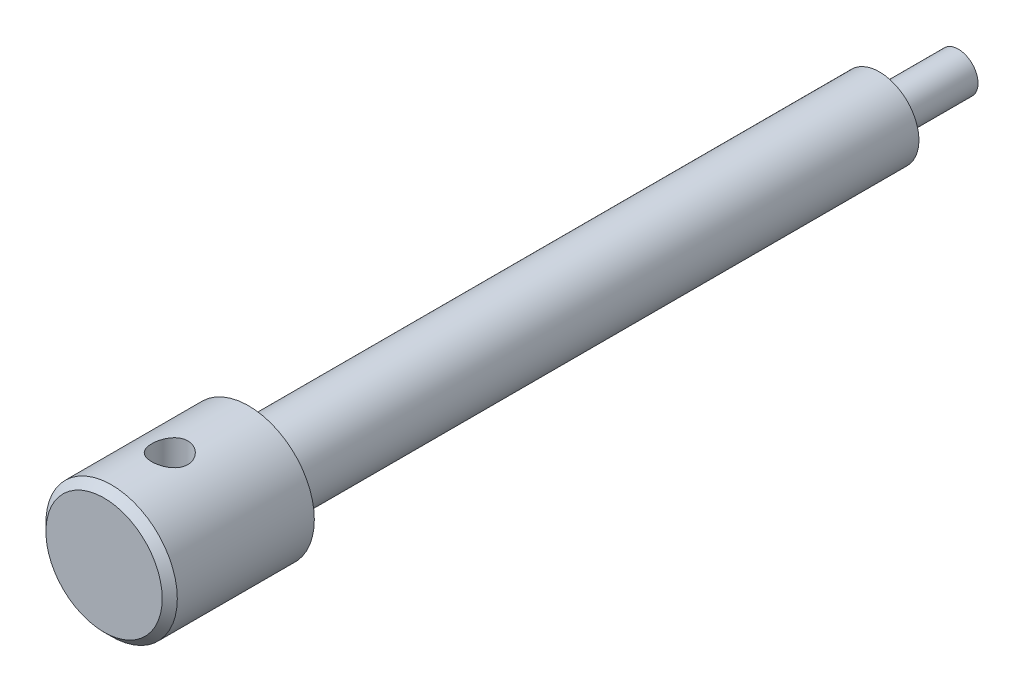
SolidWorks part; units mm, degrees
material "Plain Carbon Steel"
ref_plane "Front Plane" through (0, 0, 0) normal (0, 0, 1) x (1, 0, 0)
ref_plane "Top Plane" through (0, 0, 0) normal (0, 1, 0) x (1, 0, 0)
ref_plane "Right Plane" through (0, 0, 0) normal (1, 0, 0) x (0, 0, -1)
sketch "Head Profile Ø20" plane through (0, 0, 0) normal (0, 0, 1) x (1, 0, 0)
  circle A0 centre (0, 0) radius 10
  dimension "D1" = 20
extrude "Head Ø20x22" add sketch "Head Profile Ø20" along normal blind 22
sketch "Shank Profile Ø12" plane through (0, 0, 0) normal (0, 0, -1) x (-1, 0, 0)
  circle A0 centre (0, 0) radius 6
  dimension "D1" = 12
extrude "Threaded Shank Ø12x96" add sketch "Shank Profile Ø12" along normal blind 96
cosmetic thread "Cosmetic Thread1" parameters "D1"=90, "D2"=10.072
sketch "Pilot Profile Ø6" plane through (0, 0, -96) normal (0, 0, -1) x (-1, 0, 0)
  circle A0 centre (0, 0) radius 3
  dimension "D1" = 6
extrude "Pilot Tip Ø6x12" add sketch "Pilot Profile Ø6" along normal blind 12
sketch "Cross Hole Profile Ø5.5" plane through (0, 0, 0) normal (0, 1, 0) x (1, 0, 0)
  line L0 (10, 0) -> (-10, 0) construction
  circle A0 centre (0, -12) radius 2.75
  dimension "D2" = 5.5
  dimension "D1" = 12
extrude "Cross Hole Ø5.5" cut sketch "Cross Hole Profile Ø5.5" against normal mid plane 24
chamfer "Head Chamfer 1.15x45" distance 1.15 angle 45 1 edges at (10, 0, 22)
